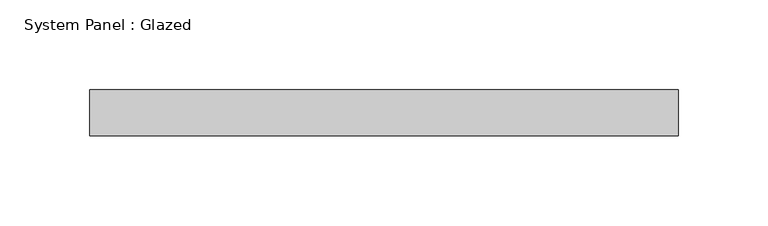
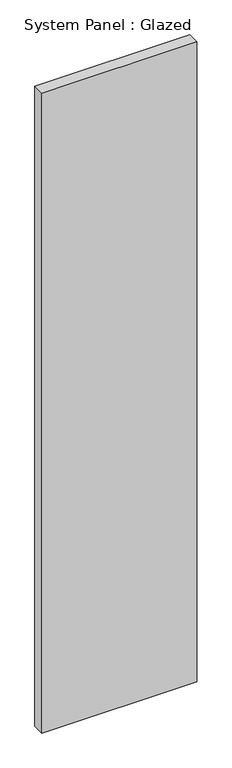
"""IFC4 building model written with IfcOpenShell, lengths in millimetres: plate geometry, System Panel : Glazed."""

from ifc_helpers import new_model, si_unit, origin, origin_with_axes, place, context, project, spatial, polyline, outline, extrude, source, transform, mapped, element, save


def system_panel_glazed_2ffdee7e(model_context):
    return source(origin(), model_context, "Body", "SweptSolid", [
        extrude(outline(polyline([(163.5125, 19.05), (-163.5125, 19.05), (-163.5125, 44.45), (163.5125, 44.45), (163.5125, 19.05)])), origin_with_axes(), (0.0, 0.0, 1.0), 1429.7181357),
    ])


if __name__ == "__main__":
    model = new_model("IFC4")
    model_context = context("Model", 3, world=origin())
    ifc_project = project(units=[si_unit("LENGTHUNIT", "METRE", prefix="MILLI")], contexts=[model_context])
    site = spatial("IfcSite", under=ifc_project)
    building = spatial("IfcBuilding", under=site)
    placement = place(None, origin())
    system_panel_glazed_shape = system_panel_glazed_2ffdee7e(model_context)
    element("IfcPlate", 1, ObjectType="System Panel : Glazed", at=placement, inside=building, context=model_context, shape_type="MappedRepresentation", body=[
        mapped(system_panel_glazed_shape, transform((0.0, 0.0, 0.0), x_axis=(1.0, 0.0, 0.0), y_axis=(0.0, 1.0, 0.0), z_axis=(0.0, 0.0, 1.0))),
    ])
    save(model, "model.ifc")

# Revit data of these elements
# Type "System Panel : Glazed"
#   Construction Type Id = "GSP4R"
#   Analytic Construction = "1/8 in Pilkington single glazing"
#   Visual Light Transmittance = 0.9
#   Solar Heat Gain Coefficient = 0.86
#   Heat Transfer Coefficient (U) = 1.18115 BTU/(h·ft²·°F)
#   Define Thermal Properties by = 1
# Element 1 (IfcPlate, "System Panel : Glazed")
#   Materials on its faces: "Glass"
# Materials
#   "Glass": class "Glass", colour RGB 0 128 192, transparency 0.75, Description = "Soda Lime Glass", Cost = 0
